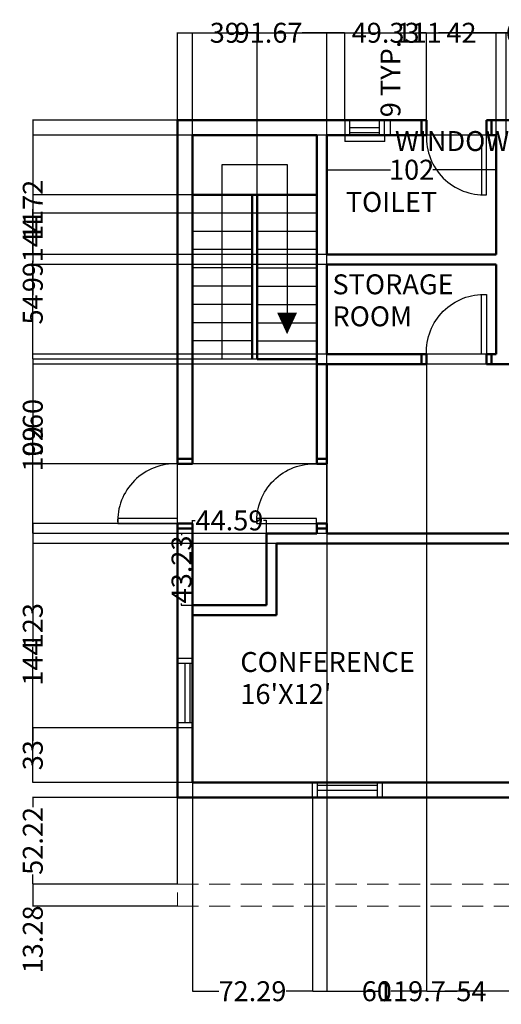
# Model space of a CAD drawing. Units: inches. Extents: x 128 to 1267, y -109 to 1208.
# Tile 1 of 8: x 128 to 418, y -90 to 503. Entities that reach past the tile are written whole.
import ezdxf

# ---------------------------------------------------------------- set-up
doc = ezdxf.new("R2010")
doc.units = ezdxf.units.IN
doc.header["$MEASUREMENT"] = 0
doc.linetypes.add('DASHED', pattern=[19.05, 12.7, -6.35])
for name, color, linetype, lineweight in [('A-ANNO-DIMS', 2, 'Continuous', 18), ('A-AREA-IDEN', 3, 'Continuous', 25), ('A-DOOR', 4, 'Continuous', 25), ('A-FLOR-STRS', 2, 'Continuous', 25), ('A-GLAZ', 3, 'Continuous', 25), ('A-ROOF-OVHD', 9, 'DASHED', 18), ('A-WALL', 7, 'Continuous', 50)]:
    doc.layers.add(name, color=color, linetype=linetype, lineweight=lineweight)
doc.styles.get("Standard").update_dxf_attribs({"font": 'arial.ttf'})
doc.dimstyles.get("Standard").update_dxf_attribs({"dimtxt": 12, "dimasz": 0.18, "dimexe": 0.18, "dimexo": 0.0625, "dimgap": 0.09, "dimtad": 0, "dimdec": 1, "dimzin": 0, "dimdsep": 46, "dimlunit": 3, "dimtxsty": 'Standard', "dimcen": 0.09, "dimadec": 0, "dimazin": 0, "dimtfac": 1, "dimtdec": 1, "dimtofl": 0, "dimtmove": 0, "dimatfit": 3, "dimfxl": 1, "dimtolj": 1, "dimtzin": 0, "dimarcsym": 0})

# ---------------------------------------------------------------- blocks, each defined once
blk = doc.blocks.new('DOOR-900')
blk.add_lwpolyline([(460.06, 187.64), (457.06, 187.64), (457.06, 151.64), (460.06, 151.64)], close=True)
blk.add_arc((458.56, 186.14), 34.53, 177.51045, 272.48955)
blk = doc.blocks.new('DOOR-875')
blk.add_lwpolyline([(592.06, 187.47), (595.06, 187.47), (595.06, 151.47), (592.06, 151.47)], close=True)
blk.add_arc((593.56, 185.98), 34.54, 267.51099, 2.76081)
blk = doc.blocks.new('WIN-900')
for p, q in [((1102.06, 345.56), (1111.06, 345.56)), ((1102.06, 342.56), (1111.06, 342.56)), ((1103.56, 306.56), (1103.56, 342.56)), ((1106.56, 306.56), (1106.56, 342.56)), ((1111.06, 306.56), (1102.06, 306.56)), ((1111.06, 303.56), (1102.06, 303.56))]:
    blk.add_line(p, q)
blk = doc.blocks.new('WIN-450')
for p, q in [((323.73, 442.64), (323.73, 433.64)), ((326.73, 442.64), (326.73, 433.64)), ((344.73, 433.64), (344.73, 442.64)), ((347.73, 433.64), (347.73, 442.64)), ((326.73, 438.14), (344.73, 438.14)), ((326.73, 435.14), (344.73, 435.14))]:
    blk.add_line(p, q)
blk = doc.blocks.new('*D14')
at = {"layer": 'A-ANNO-DIMS', "color": 0, "lineweight": -2, "transparency": 16777216}
for p, q in [((323.73, 433.58), (323.73, 429.86)), ((347.73, 433.58), (347.73, 429.86)), ((323.91, 430.04), (347.55, 430.04)), ((347.73, 430.04), (347.91, 430.04))]:
    blk.add_line(p, q, dxfattribs=at)
at = {"layer": 'A-ANNO-DIMS', "color": 0, "transparency": 16777216}
for points in [[(323.91, 430.07), (323.91, 430.01), (323.73, 430.04)], [(347.55, 430.07), (347.55, 430.01), (347.73, 430.04)]]:
    blk.add_solid(points, dxfattribs=at)
at = {"layer": 'Defpoints', "color": 0, "transparency": 16777216}
for p in [(323.73, 433.64), (347.73, 433.64), (347.73, 430.04)]:
    blk.add_point(p, dxfattribs=at)
at = {"layer": 'A-ANNO-DIMS', "color": 0, "transparency": 16777216, "insert": (431.46, 430.04), "char_height": 12, "attachment_point": 5}
blk.add_mtext('\\A1;WINDOW W2 24 TYP.', dxfattribs=at)
blk = doc.blocks.new('*D15')
at = {"layer": 'A-ANNO-DIMS', "color": 0, "lineweight": -2, "transparency": 16777216}
for p, q in [((347.79, 442.64), (351.51, 442.64)), ((351.33, 442.64), (351.33, 442.82)), ((351.33, 433.82), (351.33, 442.46)), ((347.79, 433.64), (351.51, 433.64))]:
    blk.add_line(p, q, dxfattribs=at)
at = {"layer": 'A-ANNO-DIMS', "color": 0, "transparency": 16777216}
for points in [[(351.3, 442.46), (351.36, 442.46), (351.33, 442.64)], [(351.3, 433.82), (351.36, 433.82), (351.33, 433.64)]]:
    blk.add_solid(points, dxfattribs=at)
at = {"layer": 'Defpoints', "color": 0, "transparency": 16777216}
for p in [(347.73, 442.64), (351.33, 442.64), (347.73, 433.64)]:
    blk.add_point(p, dxfattribs=at)
at = {"layer": 'A-ANNO-DIMS', "color": 0, "transparency": 16777216, "insert": (351.33, 467.45), "char_height": 12, "attachment_point": 5, "rotation": 90}
blk.add_mtext('\\A1;9 TYP.', dxfattribs=at)
blk = doc.blocks.new('*D22')
at = {"layer": 'A-ANNO-DIMS', "color": 0, "lineweight": -2, "transparency": 16777216}
for p, q in [((223.06, -17.52), (223.06, 495.44)), ((223.24, 495.26), (653.69, 495.26)), ((1110.88, 495.26), (680.42, 495.26)), ((1111.06, -17.52), (1111.06, 495.44))]:
    blk.add_line(p, q, dxfattribs=at)
at = {"layer": 'A-ANNO-DIMS', "color": 0, "transparency": 16777216}
for points in [[(223.24, 495.29), (223.24, 495.23), (223.06, 495.26)], [(1110.88, 495.29), (1110.88, 495.23), (1111.06, 495.26)]]:
    blk.add_solid(points, dxfattribs=at)
at = {"layer": 'Defpoints', "color": 0, "transparency": 16777216}
for p in [(1111.06, 495.26), (223.06, -17.58), (1111.06, -17.58)]:
    blk.add_point(p, dxfattribs=at)
at = {"layer": 'A-ANNO-DIMS', "color": 0, "transparency": 16777216, "insert": (667.06, 495.26), "char_height": 12, "attachment_point": 5}
blk.add_mtext('\\A1;888', dxfattribs=at)
blk = doc.blocks.new('*D26')
at = {"layer": 'A-ANNO-DIMS', "color": 0, "lineweight": -2, "transparency": 16777216}
for p, q in [((222.99, 34.64), (135.73, 34.64)), ((135.91, 34.46), (135.91, 28.81)), ((135.91, -17.4), (135.91, -11.75)), ((222.99, -17.58), (135.73, -17.58))]:
    blk.add_line(p, q, dxfattribs=at)
at = {"layer": 'A-ANNO-DIMS', "color": 0, "transparency": 16777216}
for points in [[(135.88, 34.46), (135.94, 34.46), (135.91, 34.64)], [(135.88, -17.4), (135.94, -17.4), (135.91, -17.58)]]:
    blk.add_solid(points, dxfattribs=at)
at = {"layer": 'Defpoints', "color": 0, "transparency": 16777216}
for p in [(223.06, 34.64), (135.91, -17.58), (223.06, -17.58)]:
    blk.add_point(p, dxfattribs=at)
at = {"layer": 'A-ANNO-DIMS', "color": 0, "transparency": 16777216, "insert": (135.91, 8.53), "char_height": 12, "attachment_point": 5, "rotation": 90}
blk.add_mtext('\\A1;52.22', dxfattribs=at)
blk = doc.blocks.new('*D27')
at = {"layer": 'A-ANNO-DIMS', "color": 0, "lineweight": -2, "transparency": 16777216}
for p, q in [((222.99, -17.58), (135.73, -17.58)), ((135.91, -17.76), (135.91, -30.68)), ((222.99, -30.86), (135.73, -30.86)), ((135.91, -30.86), (135.91, -31.04))]:
    blk.add_line(p, q, dxfattribs=at)
at = {"layer": 'A-ANNO-DIMS', "color": 0, "transparency": 16777216}
for points in [[(135.88, -17.76), (135.94, -17.76), (135.91, -17.58)], [(135.88, -30.68), (135.94, -30.68), (135.91, -30.86)]]:
    blk.add_solid(points, dxfattribs=at)
at = {"layer": 'Defpoints', "color": 0, "transparency": 16777216}
for p in [(223.06, -17.58), (135.91, -30.86), (223.06, -30.86)]:
    blk.add_point(p, dxfattribs=at)
at = {"layer": 'A-ANNO-DIMS', "color": 0, "transparency": 16777216, "insert": (135.91, -50.82), "char_height": 12, "attachment_point": 5, "rotation": 90}
blk.add_mtext('\\A1;13.28', dxfattribs=at)
blk = doc.blocks.new('*D28')
at = {"layer": 'A-ANNO-DIMS', "color": 0, "lineweight": -2, "transparency": 16777216}
for p, q in [((232.06, 43.58), (232.06, -82.19)), ((304.35, 34.58), (304.35, -82.19)), ((232.24, -82.01), (247.9, -82.01)), ((304.17, -82.01), (288.5, -82.01))]:
    blk.add_line(p, q, dxfattribs=at)
at = {"layer": 'A-ANNO-DIMS', "color": 0, "transparency": 16777216}
for points in [[(232.24, -81.98), (232.24, -82.04), (232.06, -82.01)], [(304.17, -81.98), (304.17, -82.04), (304.35, -82.01)]]:
    blk.add_solid(points, dxfattribs=at)
at = {"layer": 'Defpoints', "color": 0, "transparency": 16777216}
for p in [(232.06, 43.64), (304.35, 34.64), (304.35, -82.01)]:
    blk.add_point(p, dxfattribs=at)
at = {"layer": 'A-ANNO-DIMS', "color": 0, "transparency": 16777216, "insert": (268.2, -82.01), "char_height": 12, "attachment_point": 5}
blk.add_mtext('\\A1;72.29', dxfattribs=at)
blk = doc.blocks.new('*D29')
at = {"layer": 'A-ANNO-DIMS', "color": 0, "lineweight": -2, "transparency": 16777216}
for p, q in [((424.06, 43.58), (424.06, -82.19)), ((304.35, 34.58), (304.35, -82.19)), ((304.53, -82.01), (344.43, -82.01)), ((423.88, -82.01), (383.97, -82.01))]:
    blk.add_line(p, q, dxfattribs=at)
at = {"layer": 'A-ANNO-DIMS', "color": 0, "transparency": 16777216}
for points in [[(304.53, -81.98), (304.53, -82.04), (304.35, -82.01)], [(423.88, -81.98), (423.88, -82.04), (424.06, -82.01)]]:
    blk.add_solid(points, dxfattribs=at)
at = {"layer": 'Defpoints', "color": 0, "transparency": 16777216}
for p in [(424.06, 43.64), (304.35, 34.64), (424.06, -82.01)]:
    blk.add_point(p, dxfattribs=at)
at = {"layer": 'A-ANNO-DIMS', "color": 0, "transparency": 16777216, "insert": (364.2, -82.01), "char_height": 12, "attachment_point": 5}
blk.add_mtext('\\A1;119.7', dxfattribs=at)
blk = doc.blocks.new('*D42')
at = {"layer": 'A-ANNO-DIMS', "color": 0, "lineweight": -2, "transparency": 16777216}
for p, q in [((232.06, 433.7), (232.06, 495.44)), ((232.24, 495.26), (257.56, 495.26)), ((323.55, 495.26), (298.23, 495.26)), ((323.73, 442.7), (323.73, 495.44))]:
    blk.add_line(p, q, dxfattribs=at)
at = {"layer": 'A-ANNO-DIMS', "color": 0, "transparency": 16777216}
for points in [[(232.24, 495.29), (232.24, 495.23), (232.06, 495.26)], [(323.55, 495.29), (323.55, 495.23), (323.73, 495.26)]]:
    blk.add_solid(points, dxfattribs=at)
at = {"layer": 'Defpoints', "color": 0, "transparency": 16777216}
for p in [(323.73, 495.26), (323.73, 442.64), (232.06, 433.64)]:
    blk.add_point(p, dxfattribs=at)
at = {"layer": 'A-ANNO-DIMS', "color": 0, "transparency": 16777216, "insert": (277.89, 495.26), "char_height": 12, "attachment_point": 5}
blk.add_mtext('\\A1;91.67', dxfattribs=at)
blk = doc.blocks.new('*D43')
at = {"layer": 'A-ANNO-DIMS', "color": 0, "lineweight": -2, "transparency": 16777216}
for p, q in [((323.73, 442.7), (323.73, 495.44)), ((323.91, 495.26), (327.81, 495.26)), ((372.88, 495.26), (368.97, 495.26)), ((373.06, 442.7), (373.06, 495.44))]:
    blk.add_line(p, q, dxfattribs=at)
at = {"layer": 'A-ANNO-DIMS', "color": 0, "transparency": 16777216}
for points in [[(323.91, 495.29), (323.91, 495.23), (323.73, 495.26)], [(372.88, 495.29), (372.88, 495.23), (373.06, 495.26)]]:
    blk.add_solid(points, dxfattribs=at)
at = {"layer": 'Defpoints', "color": 0, "transparency": 16777216}
for p in [(373.06, 495.26), (323.73, 442.64), (373.06, 442.64)]:
    blk.add_point(p, dxfattribs=at)
at = {"layer": 'A-ANNO-DIMS', "color": 0, "transparency": 16777216, "insert": (348.39, 495.26), "char_height": 12, "attachment_point": 5}
blk.add_mtext('\\A1;49.33', dxfattribs=at)
blk = doc.blocks.new('*D44')
at = {"layer": 'A-ANNO-DIMS', "color": 0, "lineweight": -2, "transparency": 16777216}
for p, q in [((373.06, 442.7), (373.06, 495.44)), ((373.24, 495.26), (385.19, 495.26)), ((414.88, 495.26), (402.92, 495.26)), ((415.06, 433.7), (415.06, 495.44))]:
    blk.add_line(p, q, dxfattribs=at)
at = {"layer": 'A-ANNO-DIMS', "color": 0, "transparency": 16777216}
for points in [[(373.24, 495.29), (373.24, 495.23), (373.06, 495.26)], [(414.88, 495.29), (414.88, 495.23), (415.06, 495.26)]]:
    blk.add_solid(points, dxfattribs=at)
at = {"layer": 'Defpoints', "color": 0, "transparency": 16777216}
for p in [(415.06, 495.26), (373.06, 442.64), (415.06, 433.64)]:
    blk.add_point(p, dxfattribs=at)
at = {"layer": 'A-ANNO-DIMS', "color": 0, "transparency": 16777216, "insert": (394.06, 495.26), "char_height": 12, "attachment_point": 5}
blk.add_mtext('\\A1;42', dxfattribs=at)
blk = doc.blocks.new('*D45')
at = {"layer": 'A-ANNO-DIMS', "color": 0, "lineweight": -2, "transparency": 16777216}
for p, q in [((415.06, 433.7), (415.06, 495.44)), ((415.24, 495.26), (457.09, 495.26)), ((457.27, 442.7), (457.27, 495.44)), ((457.27, 495.26), (457.45, 495.26))]:
    blk.add_line(p, q, dxfattribs=at)
at = {"layer": 'A-ANNO-DIMS', "color": 0, "transparency": 16777216}
for points in [[(415.24, 495.29), (415.24, 495.23), (415.06, 495.26)], [(457.09, 495.29), (457.09, 495.23), (457.27, 495.26)]]:
    blk.add_solid(points, dxfattribs=at)
at = {"layer": 'Defpoints', "color": 0, "transparency": 16777216}
for p in [(457.27, 495.26), (457.27, 442.64), (415.06, 433.64)]:
    blk.add_point(p, dxfattribs=at)
at = {"layer": 'A-ANNO-DIMS', "color": 0, "transparency": 16777216, "insert": (482.67, 495.26), "char_height": 12, "attachment_point": 5}
blk.add_mtext('\\A1;42.214', dxfattribs=at)
blk = doc.blocks.new('*D56')
at = {"layer": 'A-ANNO-DIMS', "color": 0, "lineweight": -2, "transparency": 16777216}
for p, q in [((222.99, 76.64), (135.73, 76.64)), ((135.91, 76.46), (135.91, 68.82)), ((135.91, 43.82), (135.91, 51.46)), ((231.99, 43.64), (135.73, 43.64))]:
    blk.add_line(p, q, dxfattribs=at)
at = {"layer": 'A-ANNO-DIMS', "color": 0, "transparency": 16777216}
for points in [[(135.88, 76.46), (135.94, 76.46), (135.91, 76.64)], [(135.88, 43.82), (135.94, 43.82), (135.91, 43.64)]]:
    blk.add_solid(points, dxfattribs=at)
at = {"layer": 'Defpoints', "color": 0, "transparency": 16777216}
for p in [(135.91, 76.64), (223.06, 76.64), (232.06, 43.64)]:
    blk.add_point(p, dxfattribs=at)
at = {"layer": 'A-ANNO-DIMS', "color": 0, "transparency": 16777216, "insert": (135.91, 60.14), "char_height": 12, "attachment_point": 5, "rotation": 90}
blk.add_mtext('\\A1;33', dxfattribs=at)
blk = doc.blocks.new('*D57')
at = {"layer": 'A-ANNO-DIMS', "color": 0, "lineweight": -2, "transparency": 16777216}
for p, q in [((222.99, 199.64), (135.73, 199.64)), ((135.91, 199.46), (135.91, 150.92)), ((135.91, 76.82), (135.91, 125.36)), ((222.99, 76.64), (135.73, 76.64))]:
    blk.add_line(p, q, dxfattribs=at)
at = {"layer": 'A-ANNO-DIMS', "color": 0, "transparency": 16777216}
for points in [[(135.88, 199.46), (135.94, 199.46), (135.91, 199.64)], [(135.88, 76.82), (135.94, 76.82), (135.91, 76.64)]]:
    blk.add_solid(points, dxfattribs=at)
at = {"layer": 'Defpoints', "color": 0, "transparency": 16777216}
for p in [(135.91, 199.64), (223.06, 199.64), (223.06, 76.64)]:
    blk.add_point(p, dxfattribs=at)
at = {"layer": 'A-ANNO-DIMS', "color": 0, "transparency": 16777216, "insert": (135.91, 138.14), "char_height": 12, "attachment_point": 5, "rotation": 90}
blk.add_mtext('\\A1;123', dxfattribs=at)
blk = doc.blocks.new('*D58')
at = {"layer": 'A-ANNO-DIMS', "color": 0, "lineweight": -2, "transparency": 16777216}
for p, q in [((231.99, 298.64), (135.73, 298.64)), ((135.91, 298.46), (135.91, 257.84)), ((135.91, 199.82), (135.91, 240.44)), ((222.99, 199.64), (135.73, 199.64))]:
    blk.add_line(p, q, dxfattribs=at)
at = {"layer": 'A-ANNO-DIMS', "color": 0, "transparency": 16777216}
for points in [[(135.88, 298.46), (135.94, 298.46), (135.91, 298.64)], [(135.88, 199.82), (135.94, 199.82), (135.91, 199.64)]]:
    blk.add_solid(points, dxfattribs=at)
at = {"layer": 'Defpoints', "color": 0, "transparency": 16777216}
for p in [(135.91, 298.64), (232.06, 298.64), (223.06, 199.64)]:
    blk.add_point(p, dxfattribs=at)
at = {"layer": 'A-ANNO-DIMS', "color": 0, "transparency": 16777216, "insert": (135.91, 249.14), "char_height": 12, "attachment_point": 5, "rotation": 90}
blk.add_mtext('\\A1;99', dxfattribs=at)
blk = doc.blocks.new('*D59')
at = {"layer": 'A-ANNO-DIMS', "color": 0, "lineweight": -2, "transparency": 16777216}
for p, q in [((222.99, 442.64), (135.73, 442.64)), ((135.91, 442.46), (135.91, 383.4)), ((135.91, 298.82), (135.91, 357.88)), ((231.99, 298.64), (135.73, 298.64))]:
    blk.add_line(p, q, dxfattribs=at)
at = {"layer": 'A-ANNO-DIMS', "color": 0, "transparency": 16777216}
for points in [[(135.88, 442.46), (135.94, 442.46), (135.91, 442.64)], [(135.88, 298.82), (135.94, 298.82), (135.91, 298.64)]]:
    blk.add_solid(points, dxfattribs=at)
at = {"layer": 'Defpoints', "color": 0, "transparency": 16777216}
for p in [(135.91, 442.64), (223.06, 442.64), (232.06, 298.64)]:
    blk.add_point(p, dxfattribs=at)
at = {"layer": 'A-ANNO-DIMS', "color": 0, "transparency": 16777216, "insert": (135.91, 370.64), "char_height": 12, "attachment_point": 5, "rotation": 90}
blk.add_mtext('\\A1;144', dxfattribs=at)
blk = doc.blocks.new('*D64')
at = {"layer": 'A-ANNO-DIMS', "color": 0, "lineweight": -2, "transparency": 16777216}
for p, q in [((270.99, 397.64), (135.73, 397.64)), ((135.91, 397.46), (135.91, 356.84)), ((135.91, 298.82), (135.91, 339.44)), ((270.99, 298.64), (135.73, 298.64))]:
    blk.add_line(p, q, dxfattribs=at)
at = {"layer": 'A-ANNO-DIMS', "color": 0, "transparency": 16777216}
for points in [[(135.88, 397.46), (135.94, 397.46), (135.91, 397.64)], [(135.88, 298.82), (135.94, 298.82), (135.91, 298.64)]]:
    blk.add_solid(points, dxfattribs=at)
at = {"layer": 'Defpoints', "color": 0, "transparency": 16777216}
for p in [(135.91, 397.64), (271.06, 397.64), (271.06, 298.64)]:
    blk.add_point(p, dxfattribs=at)
at = {"layer": 'A-ANNO-DIMS', "color": 0, "transparency": 16777216, "insert": (135.91, 348.14), "char_height": 12, "attachment_point": 5, "rotation": 90}
blk.add_mtext('\\A1;99', dxfattribs=at)
blk = doc.blocks.new('*D66')
at = {"layer": 'A-ANNO-DIMS', "color": 0, "lineweight": -2, "transparency": 16777216}
for p, q in [((415.06, 433.7), (415.06, 495.44)), ((415.24, 495.26), (420.88, 495.26)), ((421.06, 433.7), (421.06, 495.44)), ((421.06, 495.26), (421.24, 495.26))]:
    blk.add_line(p, q, dxfattribs=at)
at = {"layer": 'A-ANNO-DIMS', "color": 0, "transparency": 16777216}
for points in [[(415.24, 495.29), (415.24, 495.23), (415.06, 495.26)], [(420.88, 495.29), (420.88, 495.23), (421.06, 495.26)]]:
    blk.add_solid(points, dxfattribs=at)
at = {"layer": 'Defpoints', "color": 0, "transparency": 16777216}
for p in [(421.06, 495.26), (415.06, 433.64), (421.06, 433.64)]:
    blk.add_point(p, dxfattribs=at)
at = {"layer": 'A-ANNO-DIMS', "color": 0, "transparency": 16777216, "insert": (425.29, 495.26), "char_height": 12, "attachment_point": 5}
blk.add_mtext('\\A1;6', dxfattribs=at)
blk = doc.blocks.new('*D67')
at = {"layer": 'A-ANNO-DIMS', "color": 0, "lineweight": -2, "transparency": 16777216}
for p, q in [((232.06, 397.7), (232.06, 495.44)), ((232.24, 495.26), (242.86, 495.26)), ((270.88, 495.26), (260.25, 495.26)), ((271.06, 397.7), (271.06, 495.44))]:
    blk.add_line(p, q, dxfattribs=at)
at = {"layer": 'A-ANNO-DIMS', "color": 0, "transparency": 16777216}
for points in [[(232.24, 495.29), (232.24, 495.23), (232.06, 495.26)], [(270.88, 495.29), (270.88, 495.23), (271.06, 495.26)]]:
    blk.add_solid(points, dxfattribs=at)
at = {"layer": 'Defpoints', "color": 0, "transparency": 16777216}
for p in [(271.06, 495.26), (232.06, 397.64), (271.06, 397.64)]:
    blk.add_point(p, dxfattribs=at)
at = {"layer": 'A-ANNO-DIMS', "color": 0, "transparency": 16777216, "insert": (251.56, 495.26), "char_height": 12, "attachment_point": 5}
blk.add_mtext('\\A1;39', dxfattribs=at)
blk = doc.blocks.new('*D68')
at = {"layer": 'A-ANNO-DIMS', "color": 0, "lineweight": -2, "transparency": 16777216}
for p, q in [((270.99, 397.64), (135.73, 397.64)), ((135.91, 397.46), (135.91, 386.82)), ((270.99, 386.64), (135.73, 386.64)), ((135.91, 386.64), (135.91, 386.46))]:
    blk.add_line(p, q, dxfattribs=at)
at = {"layer": 'A-ANNO-DIMS', "color": 0, "transparency": 16777216}
for points in [[(135.88, 397.46), (135.94, 397.46), (135.91, 397.64)], [(135.88, 386.82), (135.94, 386.82), (135.91, 386.64)]]:
    blk.add_solid(points, dxfattribs=at)
at = {"layer": 'Defpoints', "color": 0, "transparency": 16777216}
for p in [(271.06, 397.64), (135.91, 386.64), (271.06, 386.64)]:
    blk.add_point(p, dxfattribs=at)
at = {"layer": 'A-ANNO-DIMS', "color": 0, "transparency": 16777216, "insert": (135.91, 379.5), "char_height": 12, "attachment_point": 5, "rotation": 90}
blk.add_mtext('\\A1;11', dxfattribs=at)
blk = doc.blocks.new('*D69')
at = {"layer": 'A-ANNO-DIMS', "color": 0, "lineweight": -2, "transparency": 16777216}
for p, q in [((312.99, 295.64), (135.73, 295.64)), ((135.91, 295.46), (135.91, 274.34)), ((135.91, 235.82), (135.91, 256.94)), ((312.99, 235.64), (135.73, 235.64))]:
    blk.add_line(p, q, dxfattribs=at)
at = {"layer": 'A-ANNO-DIMS', "color": 0, "transparency": 16777216}
for points in [[(135.88, 295.46), (135.94, 295.46), (135.91, 295.64)], [(135.88, 235.82), (135.94, 235.82), (135.91, 235.64)]]:
    blk.add_solid(points, dxfattribs=at)
at = {"layer": 'Defpoints', "color": 0, "transparency": 16777216}
for p in [(135.91, 295.64), (313.06, 295.64), (313.06, 235.64)]:
    blk.add_point(p, dxfattribs=at)
at = {"layer": 'A-ANNO-DIMS', "color": 0, "transparency": 16777216, "insert": (135.91, 265.64), "char_height": 12, "attachment_point": 5, "rotation": 90}
blk.add_mtext('\\A1;60', dxfattribs=at)
blk = doc.blocks.new('*D70')
at = {"layer": 'A-ANNO-DIMS', "color": 0, "lineweight": -2, "transparency": 16777216}
for p, q in [((313.06, 361.7), (313.06, 412.97)), ((313.24, 412.79), (351.34, 412.79)), ((414.88, 412.79), (376.78, 412.79)), ((415.06, 361.7), (415.06, 412.97))]:
    blk.add_line(p, q, dxfattribs=at)
at = {"layer": 'A-ANNO-DIMS', "color": 0, "transparency": 16777216}
for points in [[(313.24, 412.82), (313.24, 412.76), (313.06, 412.79)], [(414.88, 412.82), (414.88, 412.76), (415.06, 412.79)]]:
    blk.add_solid(points, dxfattribs=at)
at = {"layer": 'Defpoints', "color": 0, "transparency": 16777216}
for p in [(415.06, 412.79), (313.06, 361.64), (415.06, 361.64)]:
    blk.add_point(p, dxfattribs=at)
at = {"layer": 'A-ANNO-DIMS', "color": 0, "transparency": 16777216, "insert": (364.06, 412.79), "char_height": 12, "attachment_point": 5}
blk.add_mtext('\\A1;102', dxfattribs=at)
blk = doc.blocks.new('*D71')
at = {"layer": 'A-ANNO-DIMS', "color": 0, "lineweight": -2, "transparency": 16777216}
for p, q in [((414.99, 433.64), (135.73, 433.64)), ((135.91, 433.46), (135.91, 406.21)), ((135.91, 361.82), (135.91, 389.07)), ((414.99, 361.64), (135.73, 361.64))]:
    blk.add_line(p, q, dxfattribs=at)
at = {"layer": 'A-ANNO-DIMS', "color": 0, "transparency": 16777216}
for points in [[(135.88, 433.46), (135.94, 433.46), (135.91, 433.64)], [(135.88, 361.82), (135.94, 361.82), (135.91, 361.64)]]:
    blk.add_solid(points, dxfattribs=at)
at = {"layer": 'Defpoints', "color": 0, "transparency": 16777216}
for p in [(415.06, 433.64), (135.91, 361.64), (415.06, 361.64)]:
    blk.add_point(p, dxfattribs=at)
at = {"layer": 'A-ANNO-DIMS', "color": 0, "transparency": 16777216, "insert": (135.91, 397.64), "char_height": 12, "attachment_point": 5, "rotation": 90}
blk.add_mtext('\\A1;72', dxfattribs=at)
blk = doc.blocks.new('*D72')
at = {"layer": 'A-ANNO-DIMS', "color": 0, "lineweight": -2, "transparency": 16777216}
for p, q in [((414.99, 355.64), (135.73, 355.64)), ((135.91, 355.46), (135.91, 337.3)), ((135.91, 301.82), (135.91, 319.98)), ((414.99, 301.64), (135.73, 301.64))]:
    blk.add_line(p, q, dxfattribs=at)
at = {"layer": 'A-ANNO-DIMS', "color": 0, "transparency": 16777216}
for points in [[(135.88, 355.46), (135.94, 355.46), (135.91, 355.64)], [(135.88, 301.82), (135.94, 301.82), (135.91, 301.64)]]:
    blk.add_solid(points, dxfattribs=at)
at = {"layer": 'Defpoints', "color": 0, "transparency": 16777216}
for p in [(415.06, 355.64), (135.91, 301.64), (415.06, 301.64)]:
    blk.add_point(p, dxfattribs=at)
at = {"layer": 'A-ANNO-DIMS', "color": 0, "transparency": 16777216, "insert": (135.91, 328.64), "char_height": 12, "attachment_point": 5, "rotation": 90}
blk.add_mtext('\\A1;54', dxfattribs=at)
blk = doc.blocks.new('*D74')
at = {"layer": 'A-ANNO-DIMS', "color": 0, "lineweight": -2, "transparency": 16777216}
for p, q in [((606.99, 295.64), (135.73, 295.64)), ((135.91, 295.46), (135.91, 257.36)), ((135.91, 193.82), (135.91, 231.92)), ((591.99, 193.64), (135.73, 193.64))]:
    blk.add_line(p, q, dxfattribs=at)
at = {"layer": 'A-ANNO-DIMS', "color": 0, "transparency": 16777216}
for points in [[(135.88, 295.46), (135.94, 295.46), (135.91, 295.64)], [(135.88, 193.82), (135.94, 193.82), (135.91, 193.64)]]:
    blk.add_solid(points, dxfattribs=at)
at = {"layer": 'Defpoints', "color": 0, "transparency": 16777216}
for p in [(607.06, 295.64), (135.91, 193.64), (592.06, 193.64)]:
    blk.add_point(p, dxfattribs=at)
at = {"layer": 'A-ANNO-DIMS', "color": 0, "transparency": 16777216, "insert": (135.91, 244.64), "char_height": 12, "attachment_point": 5, "rotation": 90}
blk.add_mtext('\\A1;102', dxfattribs=at)
blk = doc.blocks.new('*D75')
at = {"layer": 'A-ANNO-DIMS', "color": 0, "lineweight": -2, "transparency": 16777216}
for p, q in [((313.06, 295.58), (313.06, -82.19)), ((373.06, 295.58), (373.06, -82.19)), ((313.24, -82.01), (334.36, -82.01)), ((372.88, -82.01), (351.75, -82.01))]:
    blk.add_line(p, q, dxfattribs=at)
at = {"layer": 'A-ANNO-DIMS', "color": 0, "transparency": 16777216}
for points in [[(313.24, -81.98), (313.24, -82.04), (313.06, -82.01)], [(372.88, -81.98), (372.88, -82.04), (373.06, -82.01)]]:
    blk.add_solid(points, dxfattribs=at)
at = {"layer": 'Defpoints', "color": 0, "transparency": 16777216}
for p in [(313.06, 295.64), (373.06, 295.64), (373.06, -82.01)]:
    blk.add_point(p, dxfattribs=at)
at = {"layer": 'A-ANNO-DIMS', "color": 0, "transparency": 16777216, "insert": (343.06, -82.01), "char_height": 12, "attachment_point": 5}
blk.add_mtext('\\A1;60', dxfattribs=at)
blk = doc.blocks.new('*D76')
at = {"layer": 'A-ANNO-DIMS', "color": 0, "lineweight": -2, "transparency": 16777216}
for p, q in [((373.06, 295.58), (373.06, -82.19)), ((427.06, 295.58), (427.06, -82.19)), ((373.24, -82.01), (391.4, -82.01)), ((426.88, -82.01), (408.72, -82.01))]:
    blk.add_line(p, q, dxfattribs=at)
at = {"layer": 'A-ANNO-DIMS', "color": 0, "transparency": 16777216}
for points in [[(373.24, -81.98), (373.24, -82.04), (373.06, -82.01)], [(426.88, -81.98), (426.88, -82.04), (427.06, -82.01)]]:
    blk.add_solid(points, dxfattribs=at)
at = {"layer": 'Defpoints', "color": 0, "transparency": 16777216}
for p in [(373.06, 295.64), (427.06, 295.64), (427.06, -82.01)]:
    blk.add_point(p, dxfattribs=at)
at = {"layer": 'A-ANNO-DIMS', "color": 0, "transparency": 16777216, "insert": (400.06, -82.01), "char_height": 12, "attachment_point": 5}
blk.add_mtext('\\A1;54', dxfattribs=at)
blk = doc.blocks.new('*D79')
at = {"layer": 'A-ANNO-DIMS', "color": 0, "lineweight": -2, "transparency": 16777216}
for p, q in [((313.06, 193.7), (313.06, 495.44)), ((313.24, 495.26), (356.93, 495.26)), ((423.88, 495.26), (380.18, 495.26)), ((424.06, 193.7), (424.06, 495.44))]:
    blk.add_line(p, q, dxfattribs=at)
at = {"layer": 'A-ANNO-DIMS', "color": 0, "transparency": 16777216}
for points in [[(313.24, 495.29), (313.24, 495.23), (313.06, 495.26)], [(423.88, 495.29), (423.88, 495.23), (424.06, 495.26)]]:
    blk.add_solid(points, dxfattribs=at)
at = {"layer": 'Defpoints', "color": 0, "transparency": 16777216}
for p in [(424.06, 495.26), (313.06, 193.64), (424.06, 193.64)]:
    blk.add_point(p, dxfattribs=at)
at = {"layer": 'A-ANNO-DIMS', "color": 0, "transparency": 16777216, "insert": (368.56, 495.26), "char_height": 12, "attachment_point": 5}
blk.add_mtext('\\A1;111', dxfattribs=at)
blk = doc.blocks.new('*D83')
at = {"layer": 'A-ANNO-DIMS', "color": 0, "lineweight": -2, "transparency": 16777216}
for p, q in [((232.06, 150.47), (232.06, 201.74)), ((276.64, 150.47), (276.64, 201.74)), ((232.24, 201.56), (233.76, 201.56)), ((276.46, 201.56), (274.94, 201.56))]:
    blk.add_line(p, q, dxfattribs=at)
at = {"layer": 'A-ANNO-DIMS', "color": 0, "transparency": 16777216}
for points in [[(232.24, 201.59), (232.24, 201.53), (232.06, 201.56)], [(276.46, 201.59), (276.46, 201.53), (276.64, 201.56)]]:
    blk.add_solid(points, dxfattribs=at)
at = {"layer": 'Defpoints', "color": 0, "transparency": 16777216}
for p in [(276.64, 201.56), (232.06, 150.41), (276.64, 150.41)]:
    blk.add_point(p, dxfattribs=at)
at = {"layer": 'A-ANNO-DIMS', "color": 0, "transparency": 16777216, "insert": (254.35, 201.56), "char_height": 12, "attachment_point": 5}
blk.add_mtext('\\A1;44.59', dxfattribs=at)
blk = doc.blocks.new('*D84')
at = {"layer": 'A-ANNO-DIMS', "color": 0, "lineweight": -2, "transparency": 16777216}
for p, q in [((276.58, 193.64), (225.31, 193.64)), ((225.49, 193.46), (225.49, 192.6)), ((276.58, 150.41), (225.31, 150.41)), ((225.49, 150.59), (225.49, 151.45))]:
    blk.add_line(p, q, dxfattribs=at)
at = {"layer": 'A-ANNO-DIMS', "color": 0, "transparency": 16777216}
for points in [[(225.46, 193.46), (225.52, 193.46), (225.49, 193.64)], [(225.46, 150.59), (225.52, 150.59), (225.49, 150.41)]]:
    blk.add_solid(points, dxfattribs=at)
at = {"layer": 'Defpoints', "color": 0, "transparency": 16777216}
for p in [(225.49, 193.64), (276.64, 193.64), (276.64, 150.41)]:
    blk.add_point(p, dxfattribs=at)
at = {"layer": 'A-ANNO-DIMS', "color": 0, "transparency": 16777216, "insert": (225.49, 172.03), "char_height": 12, "attachment_point": 5, "rotation": 90}
blk.add_mtext('\\A1;43.23', dxfattribs=at)
blk = doc.blocks.new('*D85')
at = {"layer": 'A-ANNO-DIMS', "color": 0, "lineweight": -2, "transparency": 16777216}
for p, q in [((585.99, 187.64), (135.73, 187.64)), ((135.91, 187.46), (135.91, 128.4)), ((135.91, 43.82), (135.91, 102.88)), ((585.99, 43.64), (135.73, 43.64))]:
    blk.add_line(p, q, dxfattribs=at)
at = {"layer": 'A-ANNO-DIMS', "color": 0, "transparency": 16777216}
for points in [[(135.88, 187.46), (135.94, 187.46), (135.91, 187.64)], [(135.88, 43.82), (135.94, 43.82), (135.91, 43.64)]]:
    blk.add_solid(points, dxfattribs=at)
at = {"layer": 'Defpoints', "color": 0, "transparency": 16777216}
for p in [(586.06, 187.64), (135.91, 43.64), (586.06, 43.64)]:
    blk.add_point(p, dxfattribs=at)
at = {"layer": 'A-ANNO-DIMS', "color": 0, "transparency": 16777216, "insert": (135.91, 115.64), "char_height": 12, "attachment_point": 5, "rotation": 90}
blk.add_mtext('\\A1;144', dxfattribs=at)

msp = doc.modelspace()

# ---------------------------------------------------------------- linework, layer by layer
at = {"layer": 'A-FLOR-STRS'}
for p, q in [((268.056, 386.6399), (232.056, 386.6399)), ((307.056, 386.6399), (271.056, 386.6399)), ((268.056, 375.6399), (232.056, 375.6399)), ((307.056, 375.6399), (271.056, 375.6399)), ((268.056, 364.6399), (232.056, 364.6399)), ((307.056, 364.6399), (271.056, 364.6399)), ((268.056, 353.6399), (232.056, 353.6399)), ((271.056, 353.6399), (307.056, 353.6399)), ((268.056, 342.6399), (232.056, 342.6399)), ((271.056, 342.6399), (307.056, 342.6399)), ((268.056, 331.6399), (232.056, 331.6399)), ((271.056, 331.6399), (307.056, 331.6399)), ((268.056, 320.6399), (232.056, 320.6399)), ((271.056, 320.6399), (307.056, 320.6399)), ((268.056, 309.6399), (232.056, 309.6399)), ((271.056, 309.6399), (307.056, 309.6399)), ((268.056, 298.6399), (232.056, 298.6399))]:
    msp.add_line(p, q, dxfattribs=at)
msp.add_lwpolyline([(250.056, 298.6399), (250.056, 415.833), (289.056, 415.833), (289.056, 326.7)], dxfattribs=at)
msp.add_lwpolyline([(289.056, 326.7, 12, 0, 0), (289.056, 313.6774, 0, 0, 0)], format="xyseb", dxfattribs=at)
at = {"layer": 'A-ROOF-OVHD'}
for p, q in [((223.056, 34.6399), (223.056, -30.8598)), ((223.056, -17.5809), (1111.056, -17.5809)), ((223.056, -30.8598), (1111.056, -30.8598))]:
    msp.add_line(p, q, dxfattribs=at)
at = {"layer": 'A-WALL'}
for p, q in [((370.056, 433.6399), (370.056, 442.6399)), ((373.056, 433.6399), (373.056, 442.6399)), ((409.056, 433.6399), (409.056, 442.6399)), ((412.056, 433.6399), (412.056, 442.6399)), ((232.056, 433.6399), (232.056, 295.6399)), ((307.056, 433.6399), (232.056, 433.6399)), ((307.056, 433.6399), (307.056, 295.6399)), ((313.056, 433.6399), (313.056, 361.6399)), ((373.056, 433.6399), (313.056, 433.6399)), ((415.056, 433.6399), (409.056, 433.6399)), ((415.056, 433.6399), (415.056, 361.6399)), ((307.056, 397.6399), (232.056, 397.6399)), ((268.056, 397.6399), (268.056, 298.6399)), ((271.056, 397.6399), (271.056, 298.6399)), ((415.056, 361.6399), (313.056, 361.6399)), ((415.056, 355.6399), (313.056, 355.6399)), ((313.056, 355.6399), (313.056, 301.6399)), ((415.056, 355.6399), (415.056, 301.6399)), ((307.056, 298.6399), (271.056, 298.6399)), ((373.056, 301.6399), (313.056, 301.6399)), ((370.056, 301.6399), (370.056, 295.6399)), ((373.056, 301.6399), (373.056, 295.6399)), ((415.056, 301.6399), (409.056, 301.6399)), ((409.056, 301.6399), (409.056, 295.6399)), ((412.056, 301.6399), (412.056, 295.6399)), ((232.056, 295.6399), (232.056, 235.6399)), ((307.056, 295.6399), (307.056, 235.6399)), ((373.056, 295.6399), (307.056, 295.6399)), ((313.056, 295.6399), (313.056, 235.6399)), ((427.056, 295.6399), (409.056, 295.6399)), ((232.056, 271.6399), (232.056, 235.6399)), ((232.056, 238.6399), (223.056, 238.6399)), ((307.056, 238.6399), (313.056, 238.6399)), ((232.056, 235.6399), (223.056, 235.6399)), ((307.056, 235.6399), (313.056, 235.6399)), ((232.056, 199.6399), (223.056, 199.6399)), ((232.056, 196.6399), (223.056, 196.6399)), ((232.056, 199.6399), (232.056, 193.6399)), ((232.056, 199.6399), (232.056, 193.6399)), ((307.056, 199.6399), (313.056, 199.6399)), ((307.056, 199.6399), (307.056, 193.6399)), ((307.056, 196.6399), (313.056, 196.6399)), ((313.056, 199.6399), (313.056, 193.6399)), ((232.056, 193.6399), (232.056, 43.6399)), ((276.6423, 193.6399), (307.056, 193.6399)), ((276.6423, 193.6399), (276.6423, 150.4125)), ((313.056, 193.6399), (424.056, 193.6399)), ((282.6423, 187.6399), (424.056, 187.6399)), ((282.6423, 187.6399), (282.6423, 144.4125)), ((276.6423, 150.4125), (232.056, 150.4125)), ((282.6423, 144.4125), (232.056, 144.4125)), ((232.056, 43.6399), (424.056, 43.6399))]:
    msp.add_line(p, q, dxfattribs=at)
for points in [[(373.056, 442.6399), (223.056, 442.6399), (223.056, 235.6399)], [(1111.056, 427.6399), (1111.056, 442.6399), (409.056, 442.6399)], [(223.056, 199.6399), (223.056, 34.6399), (1024.056, 34.6399)]]:
    msp.add_lwpolyline(points, dxfattribs=at)

# ---------------------------------------------------------------- block references
at = {"layer": 'A-DOOR'}
msp.add_blockref('DOOR-900', (-51, 246), dxfattribs=at)
at = {"layer": 'A-DOOR', "extrusion": (0, 0, -1), "zscale": -1}
for name, p, rotation in [('DOOR-900', (51, 489.2799), 180), ('DOOR-875', (-118.3317, -392.118), 90.09796697793786)]:
    msp.add_blockref(name, p, dxfattribs=dict(at, rotation=rotation))
at = {"layer": 'A-DOOR', "rotation": 269.9999999999998}
msp.add_blockref('DOOR-900', (35.4161, 659.696), dxfattribs=at)
at = {"layer": 'A-GLAZ'}
msp.add_blockref('WIN-450', (0, 0), dxfattribs=at)
for p, rotation in [((1334.112, 422.2022), 180), ((0.7849, 1145.696), 270.0000000000005)]:
    msp.add_blockref('WIN-900', p, dxfattribs=dict(at, rotation=rotation))

# ---------------------------------------------------------------- texts
at = {"layer": 'A-AREA-IDEN'}
for s, p in [('TOILET', (324.3802, 387.3626)), ('STORAGE', (316.362, 337.7516)), ('ROOM', (316.362, 318.4747)), ('CONFERENCE', (260.9008, 110.278)), ("16'X12'", (260.9008, 91.0011))]:
    msp.add_text(s, height=12, dxfattribs=at).set_placement(p)

# ---------------------------------------------------------------- dimensions: what is measured, and where the dimension line sits
at = {"layer": 'A-ANNO-DIMS'}
for base, p1, p2, override, picture, middle in [((1111.056, 495.2611), (223.056, -17.5809), (1111.056, -17.5809), {"dimdec": 0, "dimlfac": 1, "dimrnd": 0, "dimzin": 0, "dimdsep": 46, "dimlunit": 2}, '*D22', (667.056, 495.2611)), ((323.73, 495.2611), (232.056, 433.6399), (323.73, 442.6399), {"dimdec": 2, "dimlfac": 1, "dimrnd": 0, "dimzin": 0, "dimdsep": 46, "dimlunit": 2}, '*D42', (277.893, 495.2611)), ((271.056, 495.2611), (232.056, 397.6399), (271.056, 397.6399), {"dimdec": 0, "dimlfac": 1, "dimrnd": 0, "dimzin": 0, "dimdsep": 46, "dimlunit": 2}, '*D67', (251.556, 495.2611)), ((424.056, 495.2611), (313.056, 193.6399), (424.056, 193.6399), {"dimdec": 0, "dimlfac": 1, "dimrnd": 0, "dimzin": 0, "dimdsep": 46, "dimlunit": 2}, '*D79', (368.556, 495.2611)), ((373.056, 495.2611), (323.73, 442.6399), (373.056, 442.6399), {"dimdec": 2, "dimlfac": 1, "dimrnd": 0, "dimzin": 0, "dimdsep": 46, "dimlunit": 2}, '*D43', (348.393, 495.2611)), ((415.056, 495.2611), (373.056, 442.6399), (415.056, 433.6399), {"dimdec": 0, "dimlfac": 1, "dimrnd": 0, "dimzin": 0, "dimdsep": 46, "dimlunit": 2}, '*D44', (394.056, 495.2611)), ((457.2704, 495.2611), (415.056, 433.6399), (457.2704, 442.6399), {"dimdec": 3, "dimlfac": 1, "dimrnd": 0, "dimzin": 0, "dimdsep": 46, "dimlunit": 2}, '*D45', (482.6659, 495.2611)), ((421.056, 495.2611), (415.056, 433.6399), (421.056, 433.6399), {"dimdec": 0, "dimlfac": 1, "dimrnd": 0, "dimzin": 0, "dimdsep": 46, "dimlunit": 2}, '*D66', (425.2878, 495.2611)), ((415.056, 412.7899), (313.056, 361.6399), (415.056, 361.6399), {"dimdec": 0, "dimlfac": 1, "dimrnd": 0, "dimzin": 0, "dimdsep": 46, "dimlunit": 2}, '*D70', (364.056, 412.7899)), ((373.056, -82.0098), (313.056, 295.6399), (373.056, 295.6399), {"dimdec": 0, "dimlfac": 1, "dimrnd": 0, "dimzin": 0, "dimdsep": 46, "dimlunit": 2}, '*D75', (343.056, -82.0098)), ((427.056, -82.0098), (373.056, 295.6399), (427.056, 295.6399), {"dimdec": 0, "dimlfac": 1, "dimrnd": 0, "dimzin": 0, "dimdsep": 46, "dimlunit": 2}, '*D76', (400.056, -82.0098)), ((276.6423, 201.5625), (232.056, 150.4125), (276.6423, 150.4125), {"dimdec": 2, "dimlfac": 1, "dimrnd": 0, "dimzin": 0, "dimdsep": 46, "dimlunit": 2}, '*D83', (254.3492, 201.5625)), ((304.3472, -82.0098), (232.056, 43.6399), (304.3472, 34.6399), {"dimdec": 2, "dimlfac": 1, "dimrnd": 0, "dimzin": 0, "dimdsep": 46, "dimlunit": 2}, '*D28', (268.2016, -82.0098)), ((424.056, -82.0098), (304.3472, 34.6399), (424.056, 43.6399), {"dimdec": 1, "dimlfac": 1, "dimrnd": 0, "dimzin": 0, "dimdsep": 46, "dimlunit": 2}, '*D29', (364.2016, -82.0098))]:
    dim = msp.add_linear_dim(base=base, p1=p1, p2=p2, dimstyle='Standard', override=override, dxfattribs=at)
    dim.commit()
    dim.dimension.update_dxf_attribs({"geometry": picture, "text_midpoint": middle})
dim = msp.add_linear_dim(base=(351.33, 442.6399), p1=(347.73, 433.6399), p2=(347.73, 442.6399), angle=90, text='<> TYP.', dimstyle='Standard', override={"dimdec": 0, "dimrnd": 0, "dimzin": 0, "dimlunit": 2}, dxfattribs=at)
dim.commit()
dim.dimension.update_dxf_attribs({"geometry": '*D15', "text_midpoint": (351.33, 467.4543)})
dim = msp.add_linear_dim(base=(347.73, 430.0399), p1=(323.73, 433.6399), p2=(347.73, 433.6399), text='WINDOW W2 <> TYP.', dimstyle='Standard', override={"dimdec": 0, "dimrnd": 0, "dimzin": 0, "dimlunit": 2}, dxfattribs=at)
dim.commit()
dim.dimension.update_dxf_attribs({"geometry": '*D14', "text_midpoint": (431.4598, 430.0399)})
for base, p1, p2, override, picture, middle in [((135.906, 442.6399), (232.056, 298.6399), (223.056, 442.6399), {"dimdec": 0, "dimlfac": 1, "dimrnd": 0, "dimzin": 0, "dimdsep": 46, "dimlunit": 2}, '*D59', (135.906, 370.6399)), ((135.906, 361.6399), (415.056, 433.6399), (415.056, 361.6399), {"dimdec": 0, "dimlfac": 1, "dimrnd": 0, "dimzin": 0, "dimdsep": 46, "dimlunit": 2}, '*D71', (135.906, 397.6399)), ((135.906, 397.6399), (271.056, 298.6399), (271.056, 397.6399), {"dimdec": 0, "dimlfac": 1, "dimrnd": 0, "dimzin": 0, "dimdsep": 46, "dimlunit": 2}, '*D64', (135.906, 348.1399)), ((135.906, 386.6399), (271.056, 397.6399), (271.056, 386.6399), {"dimdec": 0, "dimlfac": 1, "dimrnd": 0, "dimzin": 0, "dimdsep": 46, "dimlunit": 2}, '*D68', (135.906, 379.4982)), ((135.906, 301.6399), (415.056, 355.6399), (415.056, 301.6399), {"dimdec": 0, "dimlfac": 1, "dimrnd": 0, "dimzin": 0, "dimdsep": 46, "dimlunit": 2}, '*D72', (135.906, 328.6399)), ((135.906, 298.6399), (223.056, 199.6399), (232.056, 298.6399), {"dimdec": 0, "dimlfac": 1, "dimrnd": 0, "dimzin": 0, "dimdsep": 46, "dimlunit": 2}, '*D58', (135.906, 249.1399)), ((135.906, 295.6399), (313.056, 235.6399), (313.056, 295.6399), {"dimdec": 0, "dimlfac": 1, "dimrnd": 0, "dimzin": 0, "dimdsep": 46, "dimlunit": 2}, '*D69', (135.906, 265.6399)), ((135.906, 193.6399), (607.056, 295.6399), (592.056, 193.6399), {"dimdec": 0, "dimlfac": 1, "dimrnd": 0, "dimzin": 0, "dimdsep": 46, "dimlunit": 2}, '*D74', (135.906, 244.6399)), ((135.906, 199.6399), (223.056, 76.6399), (223.056, 199.6399), {"dimdec": 0, "dimlfac": 1, "dimrnd": 0, "dimzin": 0, "dimdsep": 46, "dimlunit": 2}, '*D57', (135.906, 138.1399)), ((225.4923, 193.6399), (276.6423, 150.4125), (276.6423, 193.6399), {"dimdec": 2, "dimlfac": 1, "dimrnd": 0, "dimzin": 0, "dimdsep": 46, "dimlunit": 2}, '*D84', (225.4923, 172.0262)), ((135.906, 43.6399), (586.056, 187.6399), (586.056, 43.6399), {"dimdec": 0, "dimlfac": 1, "dimrnd": 0, "dimzin": 0, "dimdsep": 46, "dimlunit": 2}, '*D85', (135.906, 115.6399)), ((135.906, 76.6399), (232.056, 43.6399), (223.056, 76.6399), {"dimdec": 0, "dimlfac": 1, "dimrnd": 0, "dimzin": 0, "dimdsep": 46, "dimlunit": 2}, '*D56', (135.906, 60.1399)), ((135.906, -17.5809), (223.056, 34.6399), (223.056, -17.5809), {"dimdec": 2, "dimlfac": 1, "dimrnd": 0, "dimzin": 0, "dimdsep": 46, "dimlunit": 2}, '*D26', (135.906, 8.5295)), ((135.906, -30.8598), (223.056, -17.5809), (223.056, -30.8598), {"dimdec": 2, "dimlfac": 1, "dimrnd": 0, "dimzin": 0, "dimdsep": 46, "dimlunit": 2}, '*D27', (135.906, -50.8242))]:
    dim = msp.add_linear_dim(base=base, p1=p1, p2=p2, angle=90, dimstyle='Standard', override=override, dxfattribs=at)
    dim.commit()
    dim.dimension.update_dxf_attribs({"geometry": picture, "text_midpoint": middle})

doc.saveas('drawing.dxf')
